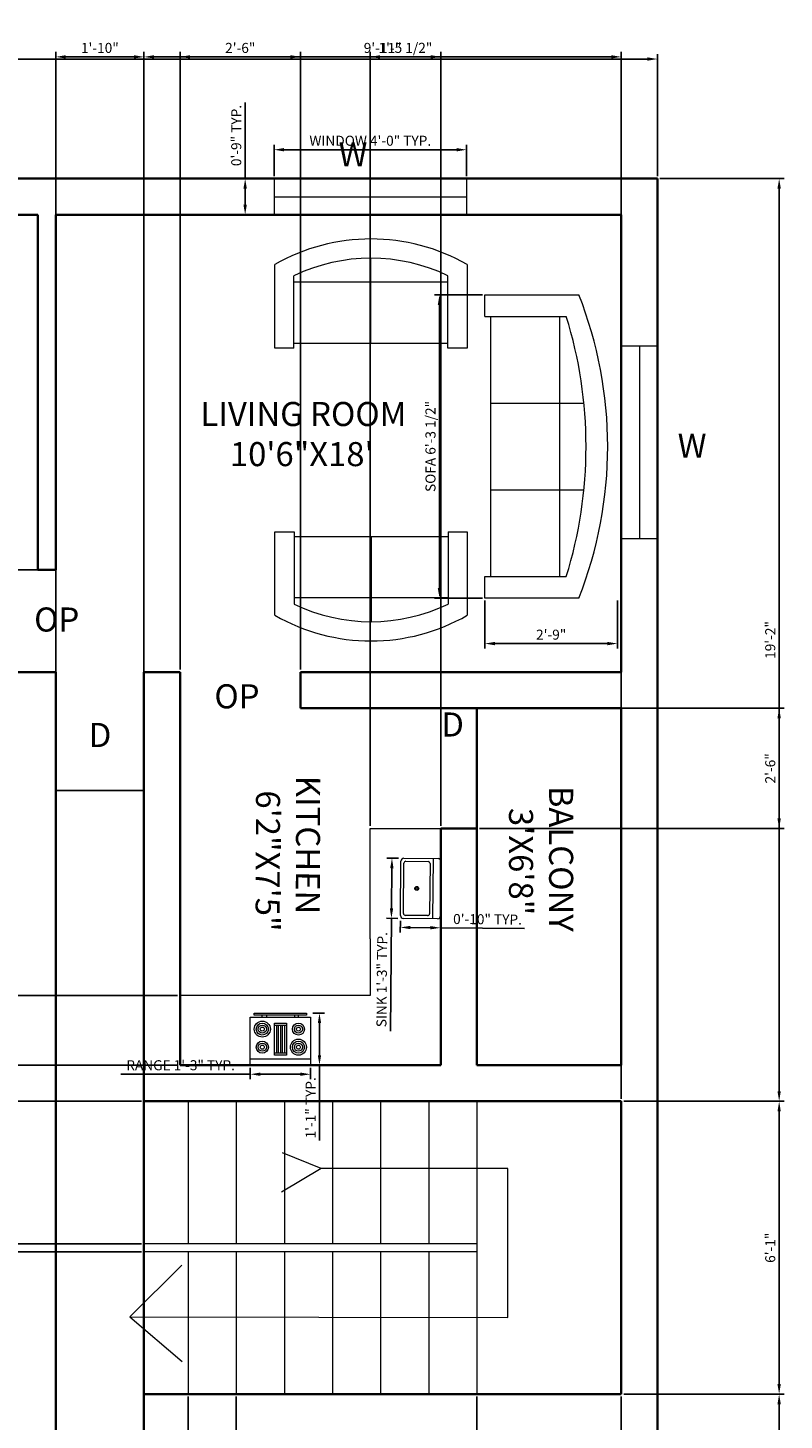
# Model space of a CAD drawing. Units: inches. Extents: x 22580 to 27643822, y 20781 to 31007121.
# Tile 3 of 3: x 27643633 to 27643822, y 31006774 to 31007121. Entities that reach past the tile are written whole.
import ezdxf

# ---------------------------------------------------------------- set-up
doc = ezdxf.new("R2010")
doc.units = ezdxf.units.IN
for name, color, linetype, lineweight in [('A-ANNO-DIMS', 2, 'Continuous', 18), ('A-ANNO-TEXT', 7, 'Continuous', 18), ('A-AREA-IDEN', 7, 'Continuous', 25), ('A-DOOR', 3, 'Continuous', 25), ('A-EQPM', 8, 'Continuous', 18), ('A-FLOR-CASE', 8, 'Continuous', 20), ('A-FLOR-FIXT', 9, 'Continuous', 18), ('A-FLOR-STRS', 7, 'Continuous', 18), ('A-FURN', 8, 'Continuous', 18), ('A-GLAZ', 4, 'Continuous', 18), ('A-WALL', 7, 'Continuous', 35)]:
    doc.layers.add(name, color=color, linetype=linetype, lineweight=lineweight)
doc.styles.get("Standard").update_dxf_attribs({"font": 'arial.ttf'})
doc.dimstyles.new('ISO-25', dxfattribs={"dimtxt": 2.5, "dimasz": 2.5, "dimexe": 1.25, "dimexo": 0.625, "dimtad": 1, "dimdec": 1, "dimlunit": 3, "dimtxsty": 'Standard', "dimcen": 2.5, "dimadec": 0, "dimazin": 0, "dimtfac": 1, "dimtdec": 1, "dimtmove": 0, "dimatfit": 3, "dimfxl": 1, "dimarcsym": 0})

# ---------------------------------------------------------------- blocks, each defined once
blk = doc.blocks.new('Sink-single - 30 in top')
blk.add_line((-15, -3.999996), (15, -3.999996))
for points in [[(-13.5, 0), (13.5, 0)], [(-15, -18.499996), (-15, -1.5)], [(-13.5, -17.499996), (-13.5, -6.499996)], [(-12.5, -5.499996), (12.5, -5.499996)], [(13.5, -6.499996), (13.5, -17.499996)], [(15, -1.5), (15, -18.499996)], [(13.5, -19.999996), (-13.5, -19.999996)], [(12.5, -18.499996), (-12.5, -18.499996)]]:
    blk.add_lwpolyline(points)
for radius in [1, 0.5]:
    blk.add_circle((0, -11.999996), radius)
for centre, radius, start, end in [((-13.5, -1.5), 1.5, 90, 180), ((-12.5, -6.499996), 1, 90, 180), ((12.5, -6.499996), 1, 0, 90), ((13.5, -1.5), 1.5, 0, 90), ((-13.5, -18.499996), 1.5, 180, 270), ((-12.5, -17.499996), 1, 180, 270), ((12.5, -17.499996), 1, 270, 0), ((13.5, -18.499996), 1.5, 270, 0)]:
    blk.add_arc(centre, radius, start, end)
blk = doc.blocks.new('Range-Oven - 30 in top')
for p, q in [((0, -3), (30, -3)), ((12, -6), (18, -6)), ((13, -20), (13, -6)), ((14, -6), (14, -20)), ((15, -20), (15, -6)), ((16, -6), (16, -20)), ((17, -20), (17, -6)), ((18, -20), (12, -20)), ((6, -24), (6, -25)), ((8, -25), (8, -24)), ((22, -25), (22, -24)), ((24, -24), (24, -25))]:
    blk.add_line(p, q)
for points in [[(0, -24), (0, 0), (30, 0), (30, -24)], [(12, -21), (12, -5), (18, -5), (18, -21)], [(2, -26), (2, -25), (28, -25), (28, -26)]]:
    blk.add_lwpolyline(points, close=True)
for centre, radius in [((6, -9), 4), ((6, -9), 3), ((24, -9), 3), ((6, -9), 2), ((6, -9), 1), ((24, -9), 2), ((24, -9), 1), ((6, -18), 3), ((6, -18), 2), ((6, -18), 1), ((24, -18), 4), ((24, -18), 3), ((24, -18), 2), ((24, -18), 1)]:
    blk.add_circle(centre, radius)
blk = doc.blocks.new('Sofa - Roundback 7 ft.')
for p, q in [((-12.00002, -32.4421), (-12.00003, -6.5971)), ((11.99997, -32.4421), (11.99998, -6.5971)), ((-36.000027, -34), (-36.000027, -11.4696)), ((35.99998, -34), (35.99998, -11.4696)), ((-35.999844, -13.3819), (35.9998, -13.3819)), ((-36.000027, -32.4421), (35.99998, -32.4421))]:
    blk.add_line(p, q)
for points in [[(-36.000027, -34), (-42.000027, -34), (-42.000027, -8)], [(41.99998, -8), (41.99998, -34), (35.99998, -34)]]:
    blk.add_lwpolyline(points)
for centre, radius, start, end in [((0, -114.25), 114.25, 68.43141, 111.5686), ((-0.00001, -127.1968), 121.1968, 72.72033, 107.2797)]:
    blk.add_arc(centre, radius, start, end)
blk = doc.blocks.new('Sofa - Roundback Loveseat 5 ft.')
for p, q in [((0, -32.44198), (0, -5.99998)), ((-24, -33.99998), (-24, -11.46958)), ((24.00004, -33.99998), (24.00004, -11.46958)), ((-23.9998, -13.38178), (23.99986, -13.38178)), ((-24, -32.44198), (24.00004, -32.44198))]:
    blk.add_line(p, q)
for points in [[(-24, -33.99998), (-30, -33.99998), (-30, -7.99998)], [(30.00004, -7.99998), (30.00004, -33.99998), (24.00004, -33.99998)]]:
    blk.add_lwpolyline(points)
for centre, radius, start, end in [((0, -60.24998), 60.24998, 60.13715, 119.8628), ((0, -61.38438), 55.38444, 64.32083, 115.6792)]:
    blk.add_arc(centre, radius, start, end)
blk = doc.blocks.new('*D9')
at = {"layer": 'A-ANNO-DIMS', "color": 0, "lineweight": -2, "transparency": 16777216}
for p, q in [((27643453.96, 31007084.46), (27643453.96, 31007114.89)), ((27643456.46, 31007113.64), (27643787.46, 31007113.64)), ((27643789.96, 31007084.46), (27643789.96, 31007114.89))]:
    blk.add_line(p, q, dxfattribs=at)
at = {"layer": 'A-ANNO-DIMS', "color": 0, "transparency": 16777216}
for points in [[(27643456.46, 31007114.06), (27643456.46, 31007113.22), (27643453.96, 31007113.64)], [(27643787.46, 31007114.06), (27643787.46, 31007113.22), (27643789.96, 31007113.64)]]:
    blk.add_solid(points, dxfattribs=at)
at = {"layer": 'Defpoints', "color": 0, "transparency": 16777216}
for p in [(27643789.96, 31007113.64), (27643453.96, 31007083.83), (27643789.96, 31007083.83)]:
    blk.add_point(p, dxfattribs=at)
at = {"layer": 'A-ANNO-DIMS', "color": 0, "transparency": 16777216, "insert": (27643621.96, 31007117.33), "char_height": 6, "attachment_point": 5}
blk.add_mtext("28'", dxfattribs=at)
blk = doc.blocks.new('WIN-48IN')
for p, q in [((0, 9), (0, 0)), ((48, 9), (48, 0)), ((0, 4.5), (48, 4.5))]:
    blk.add_line(p, q)
blk = doc.blocks.new('*D13')
at = {"layer": 'A-ANNO-DIMS', "color": 0, "lineweight": -2, "transparency": 16777216}
for p, q in [((27643694.38, 31007084.46), (27643694.38, 31007092.28)), ((27643696.88, 31007091.03), (27643739.88, 31007091.03)), ((27643742.38, 31007084.46), (27643742.38, 31007092.28))]:
    blk.add_line(p, q, dxfattribs=at)
at = {"layer": 'A-ANNO-DIMS', "color": 0, "transparency": 16777216}
for points in [[(27643696.88, 31007091.45), (27643696.88, 31007090.62), (27643694.38, 31007091.03)], [(27643739.88, 31007091.45), (27643739.88, 31007090.62), (27643742.38, 31007091.03)]]:
    blk.add_solid(points, dxfattribs=at)
at = {"layer": 'Defpoints', "color": 0, "transparency": 16777216}
for p in [(27643742.38, 31007091.03), (27643694.38, 31007083.83), (27643742.38, 31007083.83)]:
    blk.add_point(p, dxfattribs=at)
at = {"layer": 'A-ANNO-DIMS', "color": 0, "transparency": 16777216, "insert": (27643718.38, 31007092.95), "char_height": 2.5, "attachment_point": 5}
blk.add_mtext('WINDOW 4\'-0" TYP.', dxfattribs=at)
blk = doc.blocks.new('*D14')
at = {"layer": 'A-ANNO-DIMS', "color": 0, "lineweight": -2, "transparency": 16777216}
for p, q in [((27643687.18, 31007083.83), (27643687.18, 31007102.82)), ((27643693.76, 31007083.83), (27643685.93, 31007083.83)), ((27643687.18, 31007077.33), (27643687.18, 31007081.33)), ((27643693.76, 31007074.83), (27643685.93, 31007074.83))]:
    blk.add_line(p, q, dxfattribs=at)
at = {"layer": 'A-ANNO-DIMS', "color": 0, "transparency": 16777216}
for points in [[(27643686.76, 31007081.33), (27643687.6, 31007081.33), (27643687.18, 31007083.83)], [(27643686.76, 31007077.33), (27643687.6, 31007077.33), (27643687.18, 31007074.83)]]:
    blk.add_solid(points, dxfattribs=at)
at = {"layer": 'Defpoints', "color": 0, "transparency": 16777216}
for p in [(27643687.18, 31007083.83), (27643694.38, 31007083.83), (27643694.38, 31007074.83)]:
    blk.add_point(p, dxfattribs=at)
at = {"layer": 'A-ANNO-DIMS', "color": 0, "transparency": 16777216, "insert": (27643685.28, 31007094.58), "char_height": 2.5, "attachment_point": 5, "rotation": 90}
blk.add_mtext('0\'-9" TYP.', dxfattribs=at)
blk = doc.blocks.new('*D23')
at = {"layer": 'A-ANNO-DIMS', "color": 0, "lineweight": -2, "transparency": 16777216}
for p, q in [((27643746.34, 31007054.87), (27643734.38, 31007054.87)), ((27643735.63, 31007052.37), (27643735.63, 31006981.77)), ((27643746.34, 31006979.27), (27643734.38, 31006979.27))]:
    blk.add_line(p, q, dxfattribs=at)
at = {"layer": 'A-ANNO-DIMS', "color": 0, "transparency": 16777216}
for points in [[(27643735.21, 31007052.37), (27643736.05, 31007052.37), (27643735.63, 31007054.87)], [(27643735.21, 31006981.77), (27643736.05, 31006981.77), (27643735.63, 31006979.27)]]:
    blk.add_solid(points, dxfattribs=at)
at = {"layer": 'Defpoints', "color": 0, "transparency": 16777216}
for p in [(27643746.97, 31007054.87), (27643735.63, 31006979.27), (27643746.97, 31006979.27)]:
    blk.add_point(p, dxfattribs=at)
at = {"layer": 'A-ANNO-DIMS', "color": 0, "transparency": 16777216, "insert": (27643733.71, 31007017.07), "char_height": 2.5, "attachment_point": 5, "rotation": 90}
blk.add_mtext('SOFA 6\'-3 1/2"', dxfattribs=at)
blk = doc.blocks.new('*D24')
at = {"layer": 'A-ANNO-DIMS', "color": 0, "lineweight": -2, "transparency": 16777216}
for p, q in [((27643746.97, 31006978.65), (27643746.97, 31006966.68)), ((27643779.97, 31006978.65), (27643779.97, 31006966.68)), ((27643749.47, 31006967.93), (27643777.47, 31006967.93))]:
    blk.add_line(p, q, dxfattribs=at)
at = {"layer": 'A-ANNO-DIMS', "color": 0, "transparency": 16777216}
for points in [[(27643749.47, 31006968.35), (27643749.47, 31006967.51), (27643746.97, 31006967.93)], [(27643777.47, 31006968.35), (27643777.47, 31006967.51), (27643779.97, 31006967.93)]]:
    blk.add_solid(points, dxfattribs=at)
at = {"layer": 'Defpoints', "color": 0, "transparency": 16777216}
for p in [(27643746.97, 31006979.27), (27643779.97, 31006979.27), (27643779.97, 31006967.93)]:
    blk.add_point(p, dxfattribs=at)
at = {"layer": 'A-ANNO-DIMS', "color": 0, "transparency": 16777216, "insert": (27643763.47, 31006969.83), "char_height": 2.5, "attachment_point": 5}
blk.add_mtext('2\'-9"', dxfattribs=at)
blk = doc.blocks.new('*D25')
at = {"layer": 'A-ANNO-DIMS', "color": 0, "lineweight": -2, "transparency": 16777216}
for p, q in [((27643725.4, 31006914.43), (27643722.53, 31006914.46)), ((27643723.75, 31006911.95), (27643723.66, 31006901.95)), ((27643725.26, 31006899.43), (27643722.39, 31006899.46)), ((27643723.64, 31006899.45), (27643723.38, 31006871.35))]:
    blk.add_line(p, q, dxfattribs=at)
at = {"layer": 'A-ANNO-DIMS', "color": 0, "transparency": 16777216}
for points in [[(27643723.34, 31006911.95), (27643724.17, 31006911.94), (27643723.78, 31006914.44)], [(27643723.25, 31006901.95), (27643724.08, 31006901.94), (27643723.64, 31006899.45)]]:
    blk.add_solid(points, dxfattribs=at)
at = {"layer": 'Defpoints', "color": 0, "transparency": 16777216}
for p in [(27643726.03, 31006914.42), (27643723.64, 31006899.45), (27643725.89, 31006899.42)]:
    blk.add_point(p, dxfattribs=at)
at = {"layer": 'A-ANNO-DIMS', "color": 0, "transparency": 16777216, "insert": (27643721.58, 31006884.16), "char_height": 2.5, "attachment_point": 5, "rotation": 89.4746}
blk.add_mtext('SINK 1\'-3" TYP.', dxfattribs=at)
blk = doc.blocks.new('*D26')
at = {"layer": 'A-ANNO-DIMS', "color": 0, "lineweight": -2, "transparency": 16777216}
for p, q in [((27643725.88, 31006898.8), (27643725.86, 31006895.93)), ((27643728.37, 31006897.15), (27643733.37, 31006897.11)), ((27643735.88, 31006898.71), (27643735.86, 31006895.83)), ((27643735.87, 31006897.08), (27643756.8, 31006896.89))]:
    blk.add_line(p, q, dxfattribs=at)
at = {"layer": 'A-ANNO-DIMS', "color": 0, "transparency": 16777216}
for points in [[(27643728.37, 31006897.57), (27643728.36, 31006896.74), (27643725.87, 31006897.18)], [(27643733.37, 31006897.52), (27643733.36, 31006896.69), (27643735.87, 31006897.08)]]:
    blk.add_solid(points, dxfattribs=at)
at = {"layer": 'Defpoints', "color": 0, "transparency": 16777216}
for p in [(27643725.89, 31006899.42), (27643735.87, 31006897.08), (27643735.89, 31006899.33)]:
    blk.add_point(p, dxfattribs=at)
at = {"layer": 'A-ANNO-DIMS', "color": 0, "transparency": 16777216, "insert": (27643747.6, 31006898.88), "char_height": 2.5, "attachment_point": 5, "rotation": 359.4746}
blk.add_mtext('0\'-10" TYP.', dxfattribs=at)
blk = doc.blocks.new('*D27')
at = {"layer": 'A-ANNO-DIMS', "color": 0, "lineweight": -2, "transparency": 16777216}
for p, q in [((27643688.46, 31006862.21), (27643688.46, 31006859.33)), ((27643703.46, 31006862.21), (27643703.46, 31006859.33)), ((27643688.46, 31006860.58), (27643656.21, 31006860.58)), ((27643700.96, 31006860.58), (27643690.96, 31006860.58))]:
    blk.add_line(p, q, dxfattribs=at)
at = {"layer": 'A-ANNO-DIMS', "color": 0, "transparency": 16777216}
for points in [[(27643690.96, 31006861), (27643690.96, 31006860.17), (27643688.46, 31006860.58)], [(27643700.96, 31006861), (27643700.96, 31006860.17), (27643703.46, 31006860.58)]]:
    blk.add_solid(points, dxfattribs=at)
at = {"layer": 'Defpoints', "color": 0, "transparency": 16777216}
for p in [(27643688.46, 31006862.83), (27643703.46, 31006862.83), (27643688.46, 31006860.58)]:
    blk.add_point(p, dxfattribs=at)
at = {"layer": 'A-ANNO-DIMS', "color": 0, "transparency": 16777216, "insert": (27643671.08, 31006862.5), "char_height": 2.5, "attachment_point": 5}
blk.add_mtext('RANGE 1\'-3" TYP.', dxfattribs=at)
blk = doc.blocks.new('*D28')
at = {"layer": 'A-ANNO-DIMS', "color": 0, "lineweight": -2, "transparency": 16777216}
for p, q in [((27643704.08, 31006875.83), (27643706.96, 31006875.83)), ((27643705.71, 31006873.33), (27643705.71, 31006865.33)), ((27643704.08, 31006862.83), (27643706.96, 31006862.83)), ((27643705.71, 31006862.83), (27643705.71, 31006844.08))]:
    blk.add_line(p, q, dxfattribs=at)
at = {"layer": 'A-ANNO-DIMS', "color": 0, "transparency": 16777216}
for points in [[(27643705.29, 31006873.33), (27643706.12, 31006873.33), (27643705.71, 31006875.83)], [(27643705.29, 31006865.33), (27643706.12, 31006865.33), (27643705.71, 31006862.83)]]:
    blk.add_solid(points, dxfattribs=at)
at = {"layer": 'Defpoints', "color": 0, "transparency": 16777216}
for p in [(27643703.46, 31006875.83), (27643703.46, 31006862.83), (27643705.71, 31006862.83)]:
    blk.add_point(p, dxfattribs=at)
at = {"layer": 'A-ANNO-DIMS', "color": 0, "transparency": 16777216, "insert": (27643703.83, 31006852.21), "char_height": 2.5, "attachment_point": 5, "rotation": 90}
blk.add_mtext('1\'-1" TYP.', dxfattribs=at)
blk = doc.blocks.new('*D31')
at = {"layer": 'A-ANNO-DIMS', "color": 0, "lineweight": -2, "transparency": 16777216}
for p, q in [((27643661.96, 31006781.46), (27643661.96, 31007115.43)), ((27643780.96, 31006854.46), (27643780.96, 31007115.43)), ((27643664.46, 31007114.18), (27643778.46, 31007114.18))]:
    blk.add_line(p, q, dxfattribs=at)
at = {"layer": 'A-ANNO-DIMS', "color": 0, "transparency": 16777216}
for points in [[(27643664.46, 31007114.6), (27643664.46, 31007113.77), (27643661.96, 31007114.18)], [(27643778.46, 31007114.6), (27643778.46, 31007113.77), (27643780.96, 31007114.18)]]:
    blk.add_solid(points, dxfattribs=at)
at = {"layer": 'Defpoints', "color": 0, "transparency": 16777216}
for p in [(27643780.96, 31007114.18), (27643780.96, 31006853.83), (27643661.96, 31006780.83)]:
    blk.add_point(p, dxfattribs=at)
at = {"layer": 'A-ANNO-DIMS', "color": 0, "transparency": 16777216, "insert": (27643721.46, 31007116.09), "char_height": 2.5, "attachment_point": 5}
blk.add_mtext('9\'-11"', dxfattribs=at)
blk = doc.blocks.new('*D32')
at = {"layer": 'A-ANNO-DIMS', "color": 0, "lineweight": -2, "transparency": 16777216}
for p, q in [((27643781.58, 31006780.83), (27643821.56, 31006780.83)), ((27643820.31, 31006556.33), (27643820.31, 31006778.33)), ((27643790.58, 31006553.83), (27643821.56, 31006553.83))]:
    blk.add_line(p, q, dxfattribs=at)
at = {"layer": 'A-ANNO-DIMS', "color": 0, "transparency": 16777216}
for points in [[(27643819.89, 31006778.33), (27643820.72, 31006778.33), (27643820.31, 31006780.83)], [(27643819.89, 31006556.33), (27643820.72, 31006556.33), (27643820.31, 31006553.83)]]:
    blk.add_solid(points, dxfattribs=at)
at = {"layer": 'Defpoints', "color": 0, "transparency": 16777216}
for p in [(27643780.96, 31006780.83), (27643820.31, 31006780.83), (27643789.96, 31006553.83)]:
    blk.add_point(p, dxfattribs=at)
at = {"layer": 'A-ANNO-DIMS', "color": 0, "transparency": 16777216, "insert": (27643818.41, 31006667.33), "char_height": 2.5, "attachment_point": 5, "rotation": 90}
blk.add_mtext('18\'-11"', dxfattribs=at)
blk = doc.blocks.new('*D33')
at = {"layer": 'A-ANNO-DIMS', "color": 0, "lineweight": -2, "transparency": 16777216}
for p, q in [((27643781.58, 31006853.83), (27643821.56, 31006853.83)), ((27643820.31, 31006783.33), (27643820.31, 31006851.33)), ((27643781.58, 31006780.83), (27643821.56, 31006780.83))]:
    blk.add_line(p, q, dxfattribs=at)
at = {"layer": 'A-ANNO-DIMS', "color": 0, "transparency": 16777216}
for points in [[(27643819.89, 31006851.33), (27643820.72, 31006851.33), (27643820.31, 31006853.83)], [(27643819.89, 31006783.33), (27643820.72, 31006783.33), (27643820.31, 31006780.83)]]:
    blk.add_solid(points, dxfattribs=at)
at = {"layer": 'Defpoints', "color": 0, "transparency": 16777216}
for p in [(27643780.96, 31006853.83), (27643820.31, 31006853.83), (27643780.96, 31006780.83)]:
    blk.add_point(p, dxfattribs=at)
at = {"layer": 'A-ANNO-DIMS', "color": 0, "transparency": 16777216, "insert": (27643818.41, 31006817.33), "char_height": 2.5, "attachment_point": 5, "rotation": 90}
blk.add_mtext('6\'-1"', dxfattribs=at)
blk = doc.blocks.new('*D34')
at = {"layer": 'A-ANNO-DIMS', "color": 0, "lineweight": -2, "transparency": 16777216}
for p, q in [((27643790.58, 31007083.83), (27643821.56, 31007083.83)), ((27643820.31, 31006856.33), (27643820.31, 31007081.33)), ((27643781.58, 31006853.83), (27643821.56, 31006853.83))]:
    blk.add_line(p, q, dxfattribs=at)
at = {"layer": 'A-ANNO-DIMS', "color": 0, "transparency": 16777216}
for points in [[(27643819.89, 31007081.33), (27643820.72, 31007081.33), (27643820.31, 31007083.83)], [(27643819.89, 31006856.33), (27643820.72, 31006856.33), (27643820.31, 31006853.83)]]:
    blk.add_solid(points, dxfattribs=at)
at = {"layer": 'Defpoints', "color": 0, "transparency": 16777216}
for p in [(27643789.96, 31007083.83), (27643820.31, 31007083.83), (27643780.96, 31006853.83)]:
    blk.add_point(p, dxfattribs=at)
at = {"layer": 'A-ANNO-DIMS', "color": 0, "transparency": 16777216, "insert": (27643818.41, 31006968.83), "char_height": 2.5, "attachment_point": 5, "rotation": 90}
blk.add_mtext('19\'-2"', dxfattribs=at)
blk = doc.blocks.new('*D35')
at = {"layer": 'A-ANNO-DIMS', "color": 0, "lineweight": -2, "transparency": 16777216}
for p, q in [((27643639.96, 31006700.01), (27643639.96, 31007115.43)), ((27643661.96, 31006700.01), (27643661.96, 31007115.43)), ((27643642.46, 31007114.18), (27643659.46, 31007114.18))]:
    blk.add_line(p, q, dxfattribs=at)
at = {"layer": 'A-ANNO-DIMS', "color": 0, "transparency": 16777216}
for points in [[(27643642.46, 31007114.6), (27643642.46, 31007113.77), (27643639.96, 31007114.18)], [(27643659.46, 31007114.6), (27643659.46, 31007113.77), (27643661.96, 31007114.18)]]:
    blk.add_solid(points, dxfattribs=at)
at = {"layer": 'Defpoints', "color": 0, "transparency": 16777216}
for p in [(27643661.96, 31007114.18), (27643639.96, 31006699.38), (27643661.96, 31006699.38)]:
    blk.add_point(p, dxfattribs=at)
at = {"layer": 'A-ANNO-DIMS', "color": 0, "transparency": 16777216, "insert": (27643650.96, 31007116.09), "char_height": 2.5, "attachment_point": 5}
blk.add_mtext('1\'-10"', dxfattribs=at)
blk = doc.blocks.new('*D36')
at = {"layer": 'A-ANNO-DIMS', "color": 0, "lineweight": -2, "transparency": 16777216}
for p, q in [((27643744.96, 31006780.21), (27643744.96, 31006522.23)), ((27643780.96, 31006780.21), (27643780.96, 31006522.23)), ((27643747.46, 31006523.48), (27643778.46, 31006523.48))]:
    blk.add_line(p, q, dxfattribs=at)
at = {"layer": 'A-ANNO-DIMS', "color": 0, "transparency": 16777216}
for points in [[(27643747.46, 31006523.9), (27643747.46, 31006523.07), (27643744.96, 31006523.48)], [(27643778.46, 31006523.9), (27643778.46, 31006523.07), (27643780.96, 31006523.48)]]:
    blk.add_solid(points, dxfattribs=at)
at = {"layer": 'Defpoints', "color": 0, "transparency": 16777216}
for p in [(27643744.96, 31006780.83), (27643780.96, 31006780.83), (27643780.96, 31006523.48)]:
    blk.add_point(p, dxfattribs=at)
at = {"layer": 'A-ANNO-DIMS', "color": 0, "transparency": 16777216, "insert": (27643762.96, 31006525.39), "char_height": 2.5, "attachment_point": 5}
blk.add_mtext('3\'-0"', dxfattribs=at)
blk = doc.blocks.new('*D37')
at = {"layer": 'A-ANNO-DIMS', "color": 0, "lineweight": -2, "transparency": 16777216}
for p, q in [((27643672.96, 31006780.21), (27643672.96, 31006522.23)), ((27643684.96, 31006780.21), (27643684.96, 31006522.23)), ((27643675.46, 31006523.48), (27643682.46, 31006523.48))]:
    blk.add_line(p, q, dxfattribs=at)
at = {"layer": 'A-ANNO-DIMS', "color": 0, "transparency": 16777216}
for points in [[(27643675.46, 31006523.9), (27643675.46, 31006523.07), (27643672.96, 31006523.48)], [(27643682.46, 31006523.9), (27643682.46, 31006523.07), (27643684.96, 31006523.48)]]:
    blk.add_solid(points, dxfattribs=at)
at = {"layer": 'Defpoints', "color": 0, "transparency": 16777216}
for p in [(27643672.96, 31006780.83), (27643684.96, 31006780.83), (27643684.96, 31006523.48)]:
    blk.add_point(p, dxfattribs=at)
at = {"layer": 'A-ANNO-DIMS', "color": 0, "transparency": 16777216, "insert": (27643678.96, 31006525.39), "char_height": 2.5, "attachment_point": 5}
blk.add_mtext('1\'-0"', dxfattribs=at)
blk = doc.blocks.new('*D38')
at = {"layer": 'A-ANNO-DIMS', "color": 0, "lineweight": -2, "transparency": 16777216}
for p, q in [((27643661.96, 31006780.21), (27643661.96, 31006522.23)), ((27643672.96, 31006780.21), (27643672.96, 31006522.23)), ((27643664.46, 31006523.48), (27643670.46, 31006523.48))]:
    blk.add_line(p, q, dxfattribs=at)
at = {"layer": 'A-ANNO-DIMS', "color": 0, "transparency": 16777216}
for points in [[(27643664.46, 31006523.9), (27643664.46, 31006523.07), (27643661.96, 31006523.48)], [(27643670.46, 31006523.9), (27643670.46, 31006523.07), (27643672.96, 31006523.48)]]:
    blk.add_solid(points, dxfattribs=at)
at = {"layer": 'Defpoints', "color": 0, "transparency": 16777216}
for p in [(27643661.96, 31006780.83), (27643672.96, 31006780.83), (27643672.96, 31006523.48)]:
    blk.add_point(p, dxfattribs=at)
at = {"layer": 'A-ANNO-DIMS', "color": 0, "transparency": 16777216, "insert": (27643667.46, 31006525.39), "char_height": 2.5, "attachment_point": 5}
blk.add_mtext('0\'-11"', dxfattribs=at)
blk = doc.blocks.new('*D39')
at = {"layer": 'A-ANNO-DIMS', "color": 0, "lineweight": -2, "transparency": 16777216}
for p, q in [((27643661.33, 31006853.83), (27643422.36, 31006853.83)), ((27643423.61, 31006820.83), (27643423.61, 31006851.33)), ((27643661.33, 31006818.33), (27643422.36, 31006818.33))]:
    blk.add_line(p, q, dxfattribs=at)
at = {"layer": 'A-ANNO-DIMS', "color": 0, "transparency": 16777216}
for points in [[(27643423.19, 31006851.33), (27643424.02, 31006851.33), (27643423.61, 31006853.83)], [(27643423.19, 31006820.83), (27643424.02, 31006820.83), (27643423.61, 31006818.33)]]:
    blk.add_solid(points, dxfattribs=at)
at = {"layer": 'Defpoints', "color": 0, "transparency": 16777216}
for p in [(27643423.61, 31006853.83), (27643661.96, 31006853.83), (27643661.96, 31006818.33)]:
    blk.add_point(p, dxfattribs=at)
at = {"layer": 'A-ANNO-DIMS', "color": 0, "transparency": 16777216, "insert": (27643421.69, 31006836.08), "char_height": 2.5, "attachment_point": 5, "rotation": 90}
blk.add_mtext('2\'-11 1/2"', dxfattribs=at)
blk = doc.blocks.new('*D40')
at = {"layer": 'A-ANNO-DIMS', "color": 0, "lineweight": -2, "transparency": 16777216}
for p, q in [((27643423.61, 31006820.83), (27643423.61, 31006831.23)), ((27643661.33, 31006818.33), (27643422.36, 31006818.33)), ((27643423.61, 31006816.33), (27643423.61, 31006818.33)), ((27643661.33, 31006816.33), (27643422.36, 31006816.33)), ((27643423.61, 31006813.83), (27643423.61, 31006811.33))]:
    blk.add_line(p, q, dxfattribs=at)
at = {"layer": 'A-ANNO-DIMS', "color": 0, "transparency": 16777216}
for points in [[(27643423.19, 31006820.83), (27643424.02, 31006820.83), (27643423.61, 31006818.33)], [(27643423.19, 31006813.83), (27643424.02, 31006813.83), (27643423.61, 31006816.33)]]:
    blk.add_solid(points, dxfattribs=at)
at = {"layer": 'Defpoints', "color": 0, "transparency": 16777216}
for p in [(27643423.61, 31006818.33), (27643661.96, 31006818.33), (27643661.96, 31006816.33)]:
    blk.add_point(p, dxfattribs=at)
at = {"layer": 'A-ANNO-DIMS', "color": 0, "transparency": 16777216, "insert": (27643421.71, 31006827.28), "char_height": 2.5, "attachment_point": 5, "rotation": 90}
blk.add_mtext('0\'-2"', dxfattribs=at)
blk = doc.blocks.new('*D41')
at = {"layer": 'A-ANNO-DIMS', "color": 0, "lineweight": -2, "transparency": 16777216}
for p, q in [((27643670.96, 31006961.46), (27643670.96, 31007115.43)), ((27643700.96, 31006961.46), (27643700.96, 31007115.43)), ((27643673.46, 31007114.18), (27643698.46, 31007114.18))]:
    blk.add_line(p, q, dxfattribs=at)
at = {"layer": 'A-ANNO-DIMS', "color": 0, "transparency": 16777216}
for points in [[(27643673.46, 31007114.6), (27643673.46, 31007113.77), (27643670.96, 31007114.18)], [(27643698.46, 31007114.6), (27643698.46, 31007113.77), (27643700.96, 31007114.18)]]:
    blk.add_solid(points, dxfattribs=at)
at = {"layer": 'Defpoints', "color": 0, "transparency": 16777216}
for p in [(27643700.96, 31007114.18), (27643670.96, 31006960.83), (27643700.96, 31006960.83)]:
    blk.add_point(p, dxfattribs=at)
at = {"layer": 'A-ANNO-DIMS', "color": 0, "transparency": 16777216, "insert": (27643685.96, 31007116.09), "char_height": 2.5, "attachment_point": 5}
blk.add_mtext('2\'-6"', dxfattribs=at)
blk = doc.blocks.new('*D42')
at = {"layer": 'A-ANNO-DIMS', "color": 0, "lineweight": -2, "transparency": 16777216}
for p, q in [((27643745.58, 31006951.83), (27643821.56, 31006951.83)), ((27643820.31, 31006924.33), (27643820.31, 31006949.33)), ((27643745.58, 31006921.83), (27643821.56, 31006921.83))]:
    blk.add_line(p, q, dxfattribs=at)
at = {"layer": 'A-ANNO-DIMS', "color": 0, "transparency": 16777216}
for points in [[(27643819.89, 31006949.33), (27643820.72, 31006949.33), (27643820.31, 31006951.83)], [(27643819.89, 31006924.33), (27643820.72, 31006924.33), (27643820.31, 31006921.83)]]:
    blk.add_solid(points, dxfattribs=at)
at = {"layer": 'Defpoints', "color": 0, "transparency": 16777216}
for p in [(27643744.96, 31006951.83), (27643820.31, 31006951.83), (27643744.96, 31006921.83)]:
    blk.add_point(p, dxfattribs=at)
at = {"layer": 'A-ANNO-DIMS', "color": 0, "transparency": 16777216, "insert": (27643818.41, 31006936.83), "char_height": 2.5, "attachment_point": 5, "rotation": 90}
blk.add_mtext('2\'-6"', dxfattribs=at)
blk = doc.blocks.new('*D43')
at = {"layer": 'A-ANNO-DIMS', "color": 0, "lineweight": -2, "transparency": 16777216}
for p, q in [((27643670.33, 31006880.22), (27643422.36, 31006880.22)), ((27643423.61, 31006865.33), (27643423.61, 31006877.72)), ((27643670.33, 31006862.83), (27643422.36, 31006862.83))]:
    blk.add_line(p, q, dxfattribs=at)
at = {"layer": 'A-ANNO-DIMS', "color": 0, "transparency": 16777216}
for points in [[(27643423.19, 31006877.72), (27643424.02, 31006877.72), (27643423.61, 31006880.22)], [(27643423.19, 31006865.33), (27643424.02, 31006865.33), (27643423.61, 31006862.83)]]:
    blk.add_solid(points, dxfattribs=at)
at = {"layer": 'Defpoints', "color": 0, "transparency": 16777216}
for p in [(27643423.61, 31006880.22), (27643670.96, 31006880.22), (27643670.96, 31006862.83)]:
    blk.add_point(p, dxfattribs=at)
at = {"layer": 'A-ANNO-DIMS', "color": 0, "transparency": 16777216, "insert": (27643421.69, 31006871.53), "char_height": 2.5, "attachment_point": 5, "rotation": 90}
blk.add_mtext('1\'-5 1/2"', dxfattribs=at)
blk = doc.blocks.new('*D44')
at = {"layer": 'A-ANNO-DIMS', "color": 0, "lineweight": -2, "transparency": 16777216}
for p, q in [((27643718.31, 31006922.46), (27643718.31, 31007115.43)), ((27643735.96, 31006922.46), (27643735.96, 31007115.43)), ((27643720.81, 31007114.18), (27643733.46, 31007114.18))]:
    blk.add_line(p, q, dxfattribs=at)
at = {"layer": 'A-ANNO-DIMS', "color": 0, "transparency": 16777216}
for points in [[(27643720.81, 31007114.6), (27643720.81, 31007113.77), (27643718.31, 31007114.18)], [(27643733.46, 31007114.6), (27643733.46, 31007113.77), (27643735.96, 31007114.18)]]:
    blk.add_solid(points, dxfattribs=at)
at = {"layer": 'Defpoints', "color": 0, "transparency": 16777216}
for p in [(27643735.96, 31007114.18), (27643718.31, 31006921.83), (27643735.96, 31006921.83)]:
    blk.add_point(p, dxfattribs=at)
at = {"layer": 'A-ANNO-DIMS', "color": 0, "transparency": 16777216, "insert": (27643727.13, 31007116.1), "char_height": 2.5, "attachment_point": 5}
blk.add_mtext('1\'-5 1/2"', dxfattribs=at)

msp = doc.modelspace()

# ---------------------------------------------------------------- linework, layer by layer
at = {"layer": 'A-DOOR'}
for p, q in [((27643617.46, 31006986.33), (27643637.71, 31006986.33)), ((27643639.96, 31006931.32), (27643661.96, 31006931.32))]:
    msp.add_line(p, q, dxfattribs=at)
at = {"layer": 'A-FLOR-CASE'}
for p, q in [((27643718.31, 31006894.37), (27643718.31, 31006921.83)), ((27643718.31, 31006921.83), (27643735.96, 31006921.83)), ((27643718.31, 31006894.37), (27643718.31, 31006880.22)), ((27643718.31, 31006880.22), (27643670.96, 31006880.22))]:
    msp.add_line(p, q, dxfattribs=at)
at = {"layer": 'A-FLOR-STRS'}
for p, q in [((27643672.96, 31006853.83), (27643672.96, 31006818.33)), ((27643684.96, 31006853.83), (27643684.96, 31006818.33)), ((27643696.96, 31006853.83), (27643696.96, 31006818.33)), ((27643708.96, 31006853.83), (27643708.96, 31006818.33)), ((27643720.96, 31006853.83), (27643720.96, 31006818.33)), ((27643732.96, 31006853.83), (27643732.96, 31006818.33)), ((27643744.96, 31006853.83), (27643744.96, 31006780.83)), ((27643706.1, 31006837.07), (27643696.51, 31006841.01)), ((27643706.1, 31006837.07), (27643696.27, 31006831.22)), ((27643752.67, 31006837.07), (27643706.1, 31006837.07)), ((27643752.67, 31006799.91), (27643752.67, 31006837.07)), ((27643744.96, 31006818.33), (27643661.96, 31006818.33)), ((27643744.96, 31006816.33), (27643661.96, 31006816.33)), ((27643672.96, 31006816.33), (27643672.96, 31006780.83)), ((27643684.96, 31006816.33), (27643684.96, 31006780.83)), ((27643696.96, 31006816.33), (27643696.96, 31006780.83)), ((27643708.96, 31006816.33), (27643708.96, 31006780.83)), ((27643720.96, 31006816.33), (27643720.96, 31006780.83)), ((27643732.96, 31006816.33), (27643732.96, 31006780.83)), ((27643658.47, 31006800.1), (27643671.36, 31006813.03)), ((27643671.36, 31006813.03), (27643658.47, 31006800.1)), ((27643658.47, 31006800.1), (27643752.67, 31006799.91)), ((27643658.47, 31006800.1), (27643671.46, 31006788.98))]:
    msp.add_line(p, q, dxfattribs=at)
at = {"layer": 'A-WALL'}
for p, q in [((27643453.96, 31007083.83), (27643789.96, 31007083.83)), ((27643789.96, 31007083.83), (27643789.96, 31006553.83)), ((27643587.46, 31007074.83), (27643635.46, 31007074.83)), ((27643635.46, 31006986.33), (27643635.46, 31007074.83)), ((27643639.96, 31006986.33), (27643639.96, 31007074.83)), ((27643639.96, 31007074.83), (27643780.96, 31007074.83)), ((27643780.96, 31007074.83), (27643780.96, 31006960.83)), ((27643635.46, 31006986.33), (27643639.96, 31006986.33)), ((27643462.96, 31006960.83), (27643639.96, 31006960.83)), ((27643639.96, 31006670.83), (27643639.96, 31006960.83)), ((27643661.96, 31006960.83), (27643661.96, 31006853.83)), ((27643670.96, 31006960.83), (27643661.96, 31006960.83)), ((27643670.96, 31006960.83), (27643670.96, 31006862.83)), ((27643780.96, 31006960.83), (27643700.96, 31006960.83)), ((27643700.96, 31006960.83), (27643700.96, 31006951.83)), ((27643735.96, 31006951.83), (27643700.96, 31006951.83)), ((27643780.96, 31006951.83), (27643735.96, 31006951.83)), ((27643744.96, 31006951.83), (27643744.96, 31006862.83)), ((27643780.96, 31006951.83), (27643780.96, 31006862.83)), ((27643735.96, 31006921.83), (27643735.96, 31006862.83)), ((27643744.96, 31006921.83), (27643735.96, 31006921.83)), ((27643735.96, 31006862.83), (27643670.96, 31006862.83)), ((27643780.96, 31006862.83), (27643744.96, 31006862.83)), ((27643780.96, 31006853.83), (27643661.96, 31006853.83)), ((27643661.96, 31006853.83), (27643661.96, 31006682.83)), ((27643780.96, 31006853.83), (27643780.96, 31006780.83)), ((27643780.96, 31006780.83), (27643661.96, 31006780.83))]:
    msp.add_line(p, q, dxfattribs=at)

# ---------------------------------------------------------------- block references
at = {"layer": 'A-EQPM', "xscale": 0.5, "yscale": 0.5, "zscale": 0.5, "rotation": 180}
msp.add_blockref('Range-Oven - 30 in top', (27643703.46, 31006862.83), dxfattribs=at)
at = {"layer": 'A-FLOR-FIXT', "xscale": 0.5, "yscale": 0.5, "zscale": 0.5, "rotation": 269.474623121082}
msp.add_blockref('Sink-single - 30 in top', (27643735.96, 31006906.83), dxfattribs=at)
at = {"layer": 'A-FURN', "xscale": 0.8, "yscale": 0.8, "zscale": 0.8}
msp.add_blockref('Sofa - Roundback Loveseat 5 ft.', (27643718.54, 31007068.79), dxfattribs=at)
at = {"layer": 'A-FURN'}
for name, p, xscale, yscale, zscale, rotation in [('Sofa - Roundback 7 ft.', (27643777.57, 31007017.07), 0.9, 0.9, 0.5, 270), ('Sofa - Roundback Loveseat 5 ft.', (27643718.57, 31006968.59), 0.8, 0.8, 0.8, 180)]:
    msp.add_blockref(name, p, dxfattribs=dict(at, xscale=xscale, yscale=yscale, zscale=zscale, rotation=rotation))
at = {"layer": 'A-GLAZ'}
msp.add_blockref('WIN-48IN', (27643694.38, 31007074.83), dxfattribs=at)
at = {"layer": 'A-GLAZ', "rotation": 270.0000000139611}
msp.add_blockref('WIN-48IN', (27643780.96, 31007042.06), dxfattribs=at)

# ---------------------------------------------------------------- texts
at = {"layer": 'A-ANNO-TEXT', "char_height": 6, "attachment_point": 1}
for s, insert in [('W', (27643710.48, 31007092.88)), ('W', (27643795.01, 31007020.25)), ('OP', (27643634.57, 31006976.93)), ('OP', (27643679.51, 31006957.79)), (' D', (27643736.09, 31006950.76)), (' D', (27643648.19, 31006948.14))]:
    msp.add_mtext_dynamic_manual_height_columns(s, width=6.2882, gutter_width=12.5, heights=[0], dxfattribs=dict(at, insert=insert))
at = {"layer": 'A-AREA-IDEN', "insert": (27643674.21, 31007028.16), "char_height": 6, "attachment_point": 1}
msp.add_mtext_dynamic_manual_height_columns(' LIVING ROOM\\P     10\'6"X18\'', width=74.9161, gutter_width=12.5, heights=[23.22], dxfattribs=at)
at = {"layer": 'A-AREA-IDEN', "char_height": 6, "attachment_point": 1}
for s, insert, rotation in [('   KITCHEN\\P     6\'2"X7\'5"', (27643705.91, 31006940.46), 269.8273), ('    BALCONY\\P       3\'X6\'8"', (27643768.96, 31006939.8), 270)]:
    msp.add_mtext_dynamic_manual_height_columns(s, width=74.9161, gutter_width=12.5, heights=[23.22], dxfattribs=dict(at, insert=insert, rotation=rotation))

# ---------------------------------------------------------------- dimensions: what is measured, and where the dimension line sits
at = {"layer": 'A-ANNO-DIMS'}
for base, p1, p2, override, picture, middle in [((27643789.96, 31007113.64), (27643453.96, 31007083.83), (27643789.96, 31007083.83), {"dimtxt": 6, "dimclrd": 0, "dimclre": 0, "dimclrt": 0}, '*D9', (27643621.96, 31007117.33)), ((27643735.9572, 31007114.1837), (27643718.309, 31006921.8337), (27643735.9572, 31006921.8337), {"dimdec": 1, "dimlfac": 1, "dimrnd": 0, "dimzin": 1, "dimdsep": 46, "dimlunit": 4, "dimfrac": 2}, '*D44', (27643727.1331, 31007116.1013)), ((27643661.96, 31007114.18), (27643639.96, 31006699.38), (27643661.96, 31006699.38), {"dimdec": 1, "dimlfac": 1, "dimrnd": 0, "dimzin": 1, "dimdsep": 46, "dimlunit": 4, "dimfrac": 2}, '*D35', (27643650.96, 31007116.09)), ((27643780.96, 31007114.18), (27643661.96, 31006780.83), (27643780.96, 31006853.83), {"dimdec": 1, "dimlfac": 1, "dimrnd": 0, "dimzin": 1, "dimdsep": 46, "dimlunit": 4, "dimfrac": 2}, '*D31', (27643721.46, 31007116.09)), ((27643700.96, 31007114.18), (27643670.96, 31006960.83), (27643700.96, 31006960.83), {"dimdec": 1, "dimlfac": 1, "dimrnd": 0, "dimzin": 1, "dimdsep": 46, "dimlunit": 4, "dimfrac": 2}, '*D41', (27643685.96, 31007116.09)), ((27643779.97, 31006967.93), (27643746.97, 31006979.27), (27643779.97, 31006979.27), {"dimdec": 1, "dimlfac": 1, "dimrnd": 0, "dimzin": 1, "dimdsep": 46, "dimlunit": 4, "dimfrac": 2}, '*D24', (27643763.47, 31006969.83)), ((27643672.96, 31006523.48), (27643661.96, 31006780.83), (27643672.96, 31006780.83), {"dimdec": 1, "dimlfac": 1, "dimrnd": 0, "dimzin": 1, "dimdsep": 46, "dimlunit": 4, "dimfrac": 2}, '*D38', (27643667.46, 31006525.39)), ((27643684.96, 31006523.48), (27643672.96, 31006780.83), (27643684.96, 31006780.83), {"dimdec": 1, "dimlfac": 1, "dimrnd": 0, "dimzin": 1, "dimdsep": 46, "dimlunit": 4, "dimfrac": 2}, '*D37', (27643678.96, 31006525.39)), ((27643780.96, 31006523.48), (27643744.96, 31006780.83), (27643780.96, 31006780.83), {"dimdec": 1, "dimlfac": 1, "dimrnd": 0, "dimzin": 1, "dimdsep": 46, "dimlunit": 4, "dimfrac": 2}, '*D36', (27643762.96, 31006525.39))]:
    dim = msp.add_linear_dim(base=base, p1=p1, p2=p2, dimstyle='ISO-25', override=override, dxfattribs=at)
    dim.commit()
    dim.dimension.update_dxf_attribs({"geometry": picture, "text_midpoint": middle})
for base, p1, p2, angle, text, picture, middle in [((27643687.18, 31007083.83), (27643694.38, 31007074.83), (27643694.38, 31007083.83), 90, '<> TYP.', '*D14', (27643685.28, 31007094.58)), ((27643735.63, 31006979.27), (27643746.97, 31007054.87), (27643746.97, 31006979.27), 270, 'SOFA <>', '*D23', (27643733.71, 31007017.07)), ((27643723.64, 31006899.45), (27643726.03, 31006914.42), (27643725.89, 31006899.42), 269.4746, 'SINK <> TYP.', '*D25', (27643721.58, 31006884.16)), ((27643735.87, 31006897.08), (27643725.89, 31006899.42), (27643735.89, 31006899.33), 359.4746, '<> TYP.', '*D26', (27643747.6, 31006898.88)), ((27643705.71, 31006862.83), (27643703.46, 31006875.83), (27643703.46, 31006862.83), 270, '<> TYP.', '*D28', (27643703.83, 31006852.21)), ((27643688.46, 31006860.58), (27643703.46, 31006862.83), (27643688.46, 31006862.83), 180, 'RANGE <> TYP.', '*D27', (27643671.08, 31006862.5))]:
    dim = msp.add_linear_dim(base=base, p1=p1, p2=p2, angle=angle, text=text, dimstyle='ISO-25', override={"dimdec": 1, "dimlfac": 1, "dimrnd": 0, "dimzin": 1, "dimdsep": 46, "dimlunit": 4, "dimfrac": 2}, dxfattribs=at)
    dim.commit()
    dim.dimension.update_dxf_attribs({"geometry": picture, "text_midpoint": middle})
dim = msp.add_linear_dim(base=(27643742.38, 31007091.03), p1=(27643694.38, 31007083.83), p2=(27643742.38, 31007083.83), text='WINDOW <> TYP.', dimstyle='ISO-25', override={"dimdec": 1, "dimlfac": 1, "dimrnd": 0, "dimzin": 1, "dimdsep": 46, "dimlunit": 4, "dimfrac": 2}, dxfattribs=at)
dim.commit()
dim.dimension.update_dxf_attribs({"geometry": '*D13', "text_midpoint": (27643718.38, 31007092.95)})
for base, p1, p2, picture, middle in [((27643820.31, 31007083.83), (27643780.96, 31006853.83), (27643789.96, 31007083.83), '*D34', (27643818.41, 31006968.83)), ((27643820.31, 31006951.83), (27643744.96, 31006921.83), (27643744.96, 31006951.83), '*D42', (27643818.41, 31006936.83)), ((27643423.61, 31006880.22), (27643670.96, 31006862.83), (27643670.96, 31006880.22), '*D43', (27643421.69, 31006871.53)), ((27643423.61, 31006853.83), (27643661.96, 31006818.33), (27643661.96, 31006853.83), '*D39', (27643421.69, 31006836.08)), ((27643820.31, 31006853.83), (27643780.96, 31006780.83), (27643780.96, 31006853.83), '*D33', (27643818.41, 31006817.33)), ((27643423.61, 31006818.33), (27643661.96, 31006816.33), (27643661.96, 31006818.33), '*D40', (27643421.71, 31006827.28)), ((27643820.31, 31006780.83), (27643789.96, 31006553.83), (27643780.96, 31006780.83), '*D32', (27643818.41, 31006667.33))]:
    dim = msp.add_linear_dim(base=base, p1=p1, p2=p2, angle=90, dimstyle='ISO-25', override={"dimdec": 1, "dimlfac": 1, "dimrnd": 0, "dimzin": 1, "dimdsep": 46, "dimlunit": 4, "dimfrac": 2}, dxfattribs=at)
    dim.commit()
    dim.dimension.update_dxf_attribs({"geometry": picture, "text_midpoint": middle})

doc.saveas('drawing.dxf')
